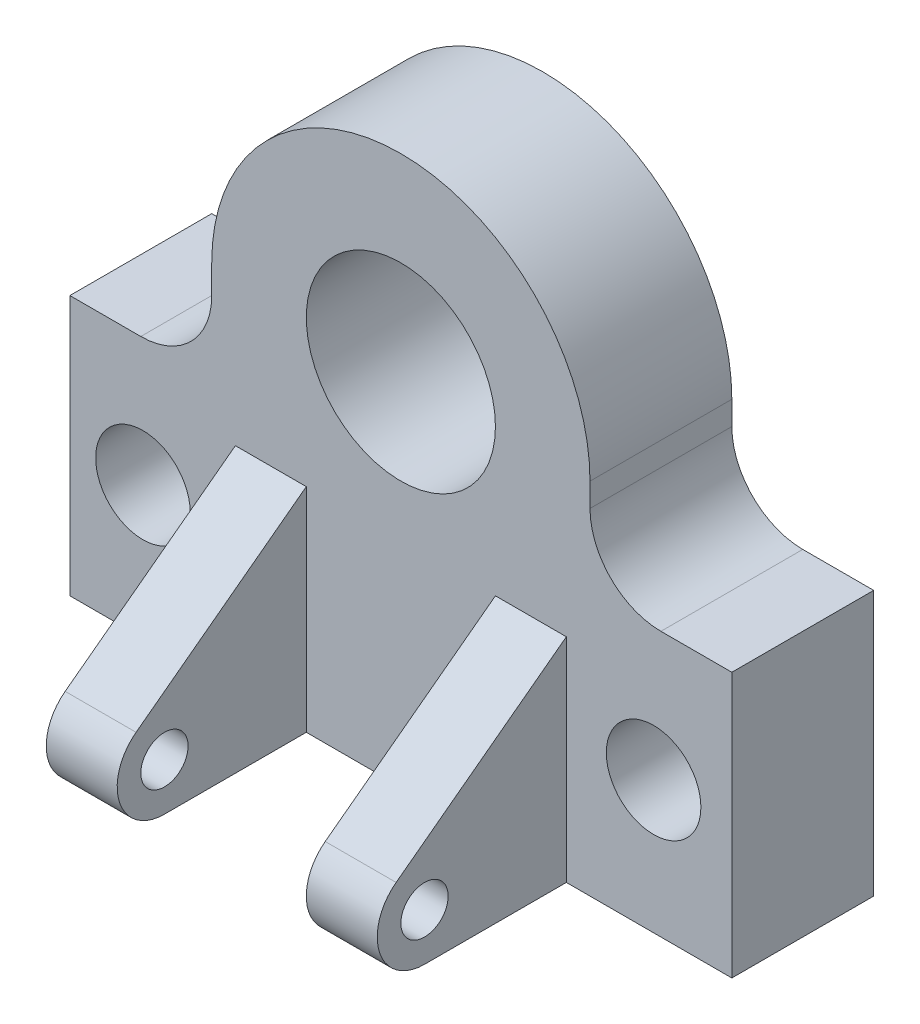
ISO-10303-21;
HEADER;
FILE_DESCRIPTION(('STEP AP214'),'2;1');
FILE_NAME('part.step','',(''),(''),'','','');
FILE_SCHEMA(('AUTOMOTIVE_DESIGN { 1 0 10303 214 1 1 1 1 }'));
ENDSEC;
DATA;
#1=APPLICATION_CONTEXT('core data for automotive mechanical design processes');
#2=APPLICATION_PROTOCOL_DEFINITION('international standard','automotive_design',2000,#1);
#3=PRODUCT_CONTEXT('',#1,'mechanical');
#4=PRODUCT('Part','Part','',(#3));
#5=PRODUCT_RELATED_PRODUCT_CATEGORY('part','',(#4));
#6=PRODUCT_DEFINITION_FORMATION('','',#4);
#7=PRODUCT_DEFINITION_CONTEXT('part definition',#1,'design');
#8=PRODUCT_DEFINITION('design','',#6,#7);
#9=PRODUCT_DEFINITION_SHAPE('','',#8);
#10=(LENGTH_UNIT() NAMED_UNIT(*) SI_UNIT(.MILLI.,.METRE.));
#11=(NAMED_UNIT(*) PLANE_ANGLE_UNIT() SI_UNIT($,.RADIAN.));
#12=(NAMED_UNIT(*) SI_UNIT($,.STERADIAN.) SOLID_ANGLE_UNIT());
#13=UNCERTAINTY_MEASURE_WITH_UNIT(LENGTH_MEASURE(1.E-05),#10,'distance_accuracy_value','');
#14=(GEOMETRIC_REPRESENTATION_CONTEXT(3) GLOBAL_UNCERTAINTY_ASSIGNED_CONTEXT((#13)) GLOBAL_UNIT_ASSIGNED_CONTEXT((#10,
#11,#12)) REPRESENTATION_CONTEXT('',''));
#15=CARTESIAN_POINT('',(0.,0.,0.));
#16=DIRECTION('',(0.,0.,1.));
#17=DIRECTION('',(1.,0.,0.));
#18=AXIS2_PLACEMENT_3D('',#15,#16,#17);
#19=CARTESIAN_POINT('',(90.,10.,60.));
#20=DIRECTION('',(1.,0.,0.));
#21=DIRECTION('',(0.,0.,-1.));
#22=AXIS2_PLACEMENT_3D('',#19,#20,#21);
#23=CYLINDRICAL_SURFACE('',#22,10.);
#24=DIRECTION('',(1.,0.,0.));
#25=VECTOR('',#24,1.);
#26=CARTESIAN_POINT('',(90.,0.,60.));
#27=LINE('',#26,#25);
#28=CARTESIAN_POINT('',(90.,0.,60.));
#29=VERTEX_POINT('',#28);
#30=CARTESIAN_POINT('',(105.,0.,60.));
#31=VERTEX_POINT('',#30);
#32=EDGE_CURVE('E179',#29,#31,#27,.T.);
#33=ORIENTED_EDGE('',*,*,#32,.T.);
#34=CARTESIAN_POINT('',(105.,10.,60.));
#35=DIRECTION('',(1.,0.,0.));
#36=DIRECTION('',(0.,0.,-1.));
#37=AXIS2_PLACEMENT_3D('',#34,#35,#36);
#38=CIRCLE('',#37,10.);
#39=CARTESIAN_POINT('',(105.,18.,66.));
#40=VERTEX_POINT('',#39);
#41=EDGE_CURVE('E167',#40,#31,#38,.T.);
#42=ORIENTED_EDGE('',*,*,#41,.F.);
#43=DIRECTION('',(1.,0.,0.));
#44=VECTOR('',#43,1.);
#45=CARTESIAN_POINT('',(90.,18.,66.));
#46=LINE('',#45,#44);
#47=CARTESIAN_POINT('',(90.,18.,66.));
#48=VERTEX_POINT('',#47);
#49=EDGE_CURVE('E178',#48,#40,#46,.T.);
#50=ORIENTED_EDGE('',*,*,#49,.F.);
#51=CARTESIAN_POINT('',(90.,10.,60.));
#52=DIRECTION('',(1.,0.,0.));
#53=DIRECTION('',(0.,0.,-1.));
#54=AXIS2_PLACEMENT_3D('',#51,#52,#53);
#55=CIRCLE('',#54,10.);
#56=EDGE_CURVE('E194',#48,#29,#55,.T.);
#57=ORIENTED_EDGE('',*,*,#56,.T.);
#58=EDGE_LOOP('',(#33,#42,#50,#57));
#59=FACE_BOUND('',#58,.T.);
#60=ADVANCED_FACE('F44',(#59),#23,.T.);
#61=CARTESIAN_POINT('',(90.,45.,30.));
#62=DIRECTION('',(0.,0.8,0.6));
#63=DIRECTION('',(0.,-0.6,0.8));
#64=AXIS2_PLACEMENT_3D('',#61,#62,#63);
#65=PLANE('',#64);
#66=ORIENTED_EDGE('',*,*,#49,.T.);
#67=DIRECTION('',(0.,-0.6,0.8));
#68=VECTOR('',#67,1.);
#69=CARTESIAN_POINT('',(105.,45.,30.));
#70=LINE('',#69,#68);
#71=CARTESIAN_POINT('',(105.,45.,30.));
#72=VERTEX_POINT('',#71);
#73=EDGE_CURVE('E170',#72,#40,#70,.T.);
#74=ORIENTED_EDGE('',*,*,#73,.F.);
#75=DIRECTION('',(1.,0.,0.));
#76=VECTOR('',#75,1.);
#77=CARTESIAN_POINT('',(90.,45.,30.));
#78=LINE('',#77,#76);
#79=CARTESIAN_POINT('',(90.,45.,30.));
#80=VERTEX_POINT('',#79);
#81=EDGE_CURVE('E190',#80,#72,#78,.T.);
#82=ORIENTED_EDGE('',*,*,#81,.F.);
#83=DIRECTION('',(0.,-0.6,0.8));
#84=VECTOR('',#83,1.);
#85=CARTESIAN_POINT('',(90.,45.,30.));
#86=LINE('',#85,#84);
#87=EDGE_CURVE('E184',#80,#48,#86,.T.);
#88=ORIENTED_EDGE('',*,*,#87,.T.);
#89=EDGE_LOOP('',(#66,#74,#82,#88));
#90=FACE_BOUND('',#89,.T.);
#91=ADVANCED_FACE('F182',(#90),#65,.T.);
#92=CARTESIAN_POINT('',(50.,10.,60.));
#93=DIRECTION('',(-1.,0.,0.));
#94=DIRECTION('',(0.,0.,1.));
#95=AXIS2_PLACEMENT_3D('',#92,#93,#94);
#96=CYLINDRICAL_SURFACE('',#95,10.);
#97=DIRECTION('',(-1.,0.,0.));
#98=VECTOR('',#97,1.);
#99=CARTESIAN_POINT('',(50.,18.,66.));
#100=LINE('',#99,#98);
#101=CARTESIAN_POINT('',(50.,18.,66.));
#102=VERTEX_POINT('',#101);
#103=CARTESIAN_POINT('',(35.,18.,66.));
#104=VERTEX_POINT('',#103);
#105=EDGE_CURVE('E232',#102,#104,#100,.T.);
#106=ORIENTED_EDGE('',*,*,#105,.T.);
#107=CARTESIAN_POINT('',(35.,10.,60.));
#108=DIRECTION('',(-1.,0.,0.));
#109=DIRECTION('',(0.,0.,1.));
#110=AXIS2_PLACEMENT_3D('',#107,#108,#109);
#111=CIRCLE('',#110,10.);
#112=CARTESIAN_POINT('',(35.,0.,60.0000000000001));
#113=VERTEX_POINT('',#112);
#114=EDGE_CURVE('E215',#113,#104,#111,.T.);
#115=ORIENTED_EDGE('',*,*,#114,.F.);
#116=DIRECTION('',(-1.,0.,0.));
#117=VECTOR('',#116,1.);
#118=CARTESIAN_POINT('',(50.,0.,60.));
#119=LINE('',#118,#117);
#120=CARTESIAN_POINT('',(50.,0.,60.));
#121=VERTEX_POINT('',#120);
#122=EDGE_CURVE('E229',#121,#113,#119,.T.);
#123=ORIENTED_EDGE('',*,*,#122,.F.);
#124=CARTESIAN_POINT('',(50.,10.,60.));
#125=DIRECTION('',(-1.,0.,0.));
#126=DIRECTION('',(0.,0.,1.));
#127=AXIS2_PLACEMENT_3D('',#124,#125,#126);
#128=CIRCLE('',#127,10.);
#129=EDGE_CURVE('E225',#121,#102,#128,.T.);
#130=ORIENTED_EDGE('',*,*,#129,.T.);
#131=EDGE_LOOP('',(#106,#115,#123,#130));
#132=FACE_BOUND('',#131,.T.);
#133=ADVANCED_FACE('F364',(#132),#96,.T.);
#134=CARTESIAN_POINT('',(50.,45.,30.));
#135=DIRECTION('',(0.,0.8,0.6));
#136=DIRECTION('',(0.,-0.6,0.8));
#137=AXIS2_PLACEMENT_3D('',#134,#135,#136);
#138=PLANE('',#137);
#139=DIRECTION('',(-1.,0.,0.));
#140=VECTOR('',#139,1.);
#141=CARTESIAN_POINT('',(50.,45.,30.));
#142=LINE('',#141,#140);
#143=CARTESIAN_POINT('',(50.,45.,30.));
#144=VERTEX_POINT('',#143);
#145=CARTESIAN_POINT('',(35.,45.,30.));
#146=VERTEX_POINT('',#145);
#147=EDGE_CURVE('E233',#144,#146,#142,.T.);
#148=ORIENTED_EDGE('',*,*,#147,.T.);
#149=DIRECTION('',(0.,0.6,-0.8));
#150=VECTOR('',#149,1.);
#151=CARTESIAN_POINT('',(35.,45.,30.));
#152=LINE('',#151,#150);
#153=EDGE_CURVE('E203',#104,#146,#152,.T.);
#154=ORIENTED_EDGE('',*,*,#153,.F.);
#155=ORIENTED_EDGE('',*,*,#105,.F.);
#156=DIRECTION('',(0.,0.6,-0.8));
#157=VECTOR('',#156,1.);
#158=CARTESIAN_POINT('',(50.,45.,30.));
#159=LINE('',#158,#157);
#160=EDGE_CURVE('E224',#102,#144,#159,.T.);
#161=ORIENTED_EDGE('',*,*,#160,.T.);
#162=EDGE_LOOP('',(#148,#154,#155,#161));
#163=FACE_BOUND('',#162,.T.);
#164=ADVANCED_FACE('F422',(#163),#138,.T.);
#165=CARTESIAN_POINT('',(0.,0.,30.));
#166=DIRECTION('',(1.,0.,0.));
#167=DIRECTION('',(0.,0.,-1.));
#168=AXIS2_PLACEMENT_3D('',#165,#166,#167);
#169=PLANE('',#168);
#170=DIRECTION('',(0.,0.,-1.));
#171=VECTOR('',#170,1.);
#172=CARTESIAN_POINT('',(0.,0.,30.));
#173=LINE('',#172,#171);
#174=CARTESIAN_POINT('',(0.,0.,30.));
#175=VERTEX_POINT('',#174);
#176=CARTESIAN_POINT('',(0.,0.,0.));
#177=VERTEX_POINT('',#176);
#178=EDGE_CURVE('E11',#175,#177,#173,.T.);
#179=ORIENTED_EDGE('',*,*,#178,.F.);
#180=DIRECTION('',(0.,-1.,0.));
#181=VECTOR('',#180,1.);
#182=CARTESIAN_POINT('',(0.,0.,30.));
#183=LINE('',#182,#181);
#184=CARTESIAN_POINT('',(0.,55.,30.));
#185=VERTEX_POINT('',#184);
#186=EDGE_CURVE('E251',#185,#175,#183,.T.);
#187=ORIENTED_EDGE('',*,*,#186,.F.);
#188=DIRECTION('',(0.,0.,-1.));
#189=VECTOR('',#188,1.);
#190=CARTESIAN_POINT('',(0.,55.,30.));
#191=LINE('',#190,#189);
#192=CARTESIAN_POINT('',(0.,55.,0.));
#193=VERTEX_POINT('',#192);
#194=EDGE_CURVE('E273',#185,#193,#191,.T.);
#195=ORIENTED_EDGE('',*,*,#194,.T.);
#196=DIRECTION('',(0.,-1.,0.));
#197=VECTOR('',#196,1.);
#198=CARTESIAN_POINT('',(0.,0.,0.));
#199=LINE('',#198,#197);
#200=EDGE_CURVE('E252',#193,#177,#199,.T.);
#201=ORIENTED_EDGE('',*,*,#200,.T.);
#202=EDGE_LOOP('',(#179,#187,#195,#201));
#203=FACE_BOUND('',#202,.T.);
#204=ADVANCED_FACE('F50',(#203),#169,.F.);
#205=CARTESIAN_POINT('',(0.,0.,30.));
#206=DIRECTION('',(0.,1.,0.));
#207=DIRECTION('',(0.,0.,1.));
#208=AXIS2_PLACEMENT_3D('',#205,#206,#207);
#209=PLANE('',#208);
#210=DIRECTION('',(0.,0.,-1.));
#211=VECTOR('',#210,1.);
#212=CARTESIAN_POINT('',(140.,0.,30.));
#213=LINE('',#212,#211);
#214=CARTESIAN_POINT('',(140.,0.,30.));
#215=VERTEX_POINT('',#214);
#216=CARTESIAN_POINT('',(140.,0.,0.));
#217=VERTEX_POINT('',#216);
#218=EDGE_CURVE('E52',#215,#217,#213,.T.);
#219=ORIENTED_EDGE('',*,*,#218,.F.);
#220=DIRECTION('',(1.,0.,0.));
#221=VECTOR('',#220,1.);
#222=CARTESIAN_POINT('',(105.,0.,30.));
#223=LINE('',#222,#221);
#224=CARTESIAN_POINT('',(105.,0.,30.));
#225=VERTEX_POINT('',#224);
#226=EDGE_CURVE('E198',#225,#215,#223,.T.);
#227=ORIENTED_EDGE('',*,*,#226,.F.);
#228=DIRECTION('',(0.,0.,-1.));
#229=VECTOR('',#228,1.);
#230=CARTESIAN_POINT('',(105.,0.,30.));
#231=LINE('',#230,#229);
#232=EDGE_CURVE('E181',#31,#225,#231,.T.);
#233=ORIENTED_EDGE('',*,*,#232,.F.);
#234=ORIENTED_EDGE('',*,*,#32,.F.);
#235=DIRECTION('',(0.,0.,-1.));
#236=VECTOR('',#235,1.);
#237=CARTESIAN_POINT('',(90.,0.,30.));
#238=LINE('',#237,#236);
#239=CARTESIAN_POINT('',(90.,0.,30.));
#240=VERTEX_POINT('',#239);
#241=EDGE_CURVE('E197',#29,#240,#238,.T.);
#242=ORIENTED_EDGE('',*,*,#241,.T.);
#243=DIRECTION('',(1.,0.,0.));
#244=VECTOR('',#243,1.);
#245=CARTESIAN_POINT('',(0.,0.,30.));
#246=LINE('',#245,#244);
#247=CARTESIAN_POINT('',(50.,0.,30.));
#248=VERTEX_POINT('',#247);
#249=EDGE_CURVE('E259',#248,#240,#246,.T.);
#250=ORIENTED_EDGE('',*,*,#249,.F.);
#251=DIRECTION('',(0.,0.,1.));
#252=VECTOR('',#251,1.);
#253=CARTESIAN_POINT('',(50.,0.,30.));
#254=LINE('',#253,#252);
#255=EDGE_CURVE('E218',#248,#121,#254,.T.);
#256=ORIENTED_EDGE('',*,*,#255,.T.);
#257=ORIENTED_EDGE('',*,*,#122,.T.);
#258=DIRECTION('',(0.,0.,1.));
#259=VECTOR('',#258,1.);
#260=CARTESIAN_POINT('',(35.,0.,30.));
#261=LINE('',#260,#259);
#262=CARTESIAN_POINT('',(35.,0.,30.));
#263=VERTEX_POINT('',#262);
#264=EDGE_CURVE('E214',#263,#113,#261,.T.);
#265=ORIENTED_EDGE('',*,*,#264,.F.);
#266=DIRECTION('',(-1.,0.,0.));
#267=VECTOR('',#266,1.);
#268=CARTESIAN_POINT('',(35.,0.,30.));
#269=LINE('',#268,#267);
#270=EDGE_CURVE('E212',#263,#175,#269,.T.);
#271=ORIENTED_EDGE('',*,*,#270,.T.);
#272=ORIENTED_EDGE('',*,*,#178,.T.);
#273=DIRECTION('',(1.,0.,0.));
#274=VECTOR('',#273,1.);
#275=CARTESIAN_POINT('',(0.,0.,0.));
#276=LINE('',#275,#274);
#277=EDGE_CURVE('E280',#177,#217,#276,.T.);
#278=ORIENTED_EDGE('',*,*,#277,.T.);
#279=EDGE_LOOP('',(#219,#227,#233,#234,#242,#250,#256,#257,#265,#271,#272,#278));
#280=FACE_BOUND('',#279,.T.);
#281=ADVANCED_FACE('F330',(#280),#209,.F.);
#282=CARTESIAN_POINT('',(140.,0.,30.));
#283=DIRECTION('',(-1.,0.,0.));
#284=DIRECTION('',(0.,0.,1.));
#285=AXIS2_PLACEMENT_3D('',#282,#283,#284);
#286=PLANE('',#285);
#287=DIRECTION('',(0.,1.,0.));
#288=VECTOR('',#287,1.);
#289=CARTESIAN_POINT('',(140.,0.,30.));
#290=LINE('',#289,#288);
#291=CARTESIAN_POINT('',(140.,56.,30.));
#292=VERTEX_POINT('',#291);
#293=EDGE_CURVE('E258',#215,#292,#290,.T.);
#294=ORIENTED_EDGE('',*,*,#293,.F.);
#295=ORIENTED_EDGE('',*,*,#218,.T.);
#296=DIRECTION('',(0.,1.,0.));
#297=VECTOR('',#296,1.);
#298=CARTESIAN_POINT('',(140.,0.,0.));
#299=LINE('',#298,#297);
#300=CARTESIAN_POINT('',(140.,56.,0.));
#301=VERTEX_POINT('',#300);
#302=EDGE_CURVE('E281',#217,#301,#299,.T.);
#303=ORIENTED_EDGE('',*,*,#302,.T.);
#304=DIRECTION('',(0.,0.,-1.));
#305=VECTOR('',#304,1.);
#306=CARTESIAN_POINT('',(140.,56.,30.));
#307=LINE('',#306,#305);
#308=EDGE_CURVE('E317',#292,#301,#307,.T.);
#309=ORIENTED_EDGE('',*,*,#308,.F.);
#310=EDGE_LOOP('',(#294,#295,#303,#309));
#311=FACE_BOUND('',#310,.T.);
#312=ADVANCED_FACE('F318',(#311),#286,.F.);
#313=CARTESIAN_POINT('',(140.,56.,30.));
#314=DIRECTION('',(0.,-1.,0.));
#315=DIRECTION('',(0.,0.,-1.));
#316=AXIS2_PLACEMENT_3D('',#313,#314,#315);
#317=PLANE('',#316);
#318=DIRECTION('',(-1.,0.,0.));
#319=VECTOR('',#318,1.);
#320=CARTESIAN_POINT('',(140.,56.,0.));
#321=LINE('',#320,#319);
#322=CARTESIAN_POINT('',(125.,56.,0.));
#323=VERTEX_POINT('',#322);
#324=EDGE_CURVE('E282',#301,#323,#321,.T.);
#325=ORIENTED_EDGE('',*,*,#324,.T.);
#326=DIRECTION('',(0.,0.,-1.));
#327=VECTOR('',#326,1.);
#328=CARTESIAN_POINT('',(125.,56.,30.));
#329=LINE('',#328,#327);
#330=CARTESIAN_POINT('',(125.,56.,30.));
#331=VERTEX_POINT('',#330);
#332=EDGE_CURVE('E312',#331,#323,#329,.T.);
#333=ORIENTED_EDGE('',*,*,#332,.F.);
#334=DIRECTION('',(-1.,0.,0.));
#335=VECTOR('',#334,1.);
#336=CARTESIAN_POINT('',(140.,56.,30.));
#337=LINE('',#336,#335);
#338=EDGE_CURVE('E261',#292,#331,#337,.T.);
#339=ORIENTED_EDGE('',*,*,#338,.F.);
#340=ORIENTED_EDGE('',*,*,#308,.T.);
#341=EDGE_LOOP('',(#325,#333,#339,#340));
#342=FACE_BOUND('',#341,.T.);
#343=ADVANCED_FACE('F340',(#342),#317,.F.);
#344=CARTESIAN_POINT('',(125.,71.,30.));
#345=DIRECTION('',(0.,0.,-1.));
#346=DIRECTION('',(-1.,0.,0.));
#347=AXIS2_PLACEMENT_3D('',#344,#345,#346);
#348=CYLINDRICAL_SURFACE('',#347,15.);
#349=CARTESIAN_POINT('',(125.,71.,0.));
#350=DIRECTION('',(0.,0.,-1.));
#351=DIRECTION('',(1.,0.,0.));
#352=AXIS2_PLACEMENT_3D('',#349,#350,#351);
#353=CIRCLE('',#352,15.);
#354=CARTESIAN_POINT('',(110.,71.,0.));
#355=VERTEX_POINT('',#354);
#356=EDGE_CURVE('E284',#323,#355,#353,.T.);
#357=ORIENTED_EDGE('',*,*,#356,.T.);
#358=DIRECTION('',(0.,0.,-1.));
#359=VECTOR('',#358,1.);
#360=CARTESIAN_POINT('',(110.,71.,30.));
#361=LINE('',#360,#359);
#362=CARTESIAN_POINT('',(110.,71.,30.));
#363=VERTEX_POINT('',#362);
#364=EDGE_CURVE('E309',#363,#355,#361,.T.);
#365=ORIENTED_EDGE('',*,*,#364,.F.);
#366=CARTESIAN_POINT('',(125.,71.,30.));
#367=DIRECTION('',(0.,0.,-1.));
#368=DIRECTION('',(1.,0.,0.));
#369=AXIS2_PLACEMENT_3D('',#366,#367,#368);
#370=CIRCLE('',#369,15.);
#371=EDGE_CURVE('E262',#331,#363,#370,.T.);
#372=ORIENTED_EDGE('',*,*,#371,.F.);
#373=ORIENTED_EDGE('',*,*,#332,.T.);
#374=EDGE_LOOP('',(#357,#365,#372,#373));
#375=FACE_BOUND('',#374,.T.);
#376=ADVANCED_FACE('F344',(#375),#348,.F.);
#377=CARTESIAN_POINT('',(110.,76.,30.));
#378=DIRECTION('',(-1.,0.,0.));
#379=DIRECTION('',(0.,0.,1.));
#380=AXIS2_PLACEMENT_3D('',#377,#378,#379);
#381=PLANE('',#380);
#382=DIRECTION('',(0.,1.,0.));
#383=VECTOR('',#382,1.);
#384=CARTESIAN_POINT('',(110.,76.,0.));
#385=LINE('',#384,#383);
#386=CARTESIAN_POINT('',(110.,76.,0.));
#387=VERTEX_POINT('',#386);
#388=EDGE_CURVE('E290',#355,#387,#385,.T.);
#389=ORIENTED_EDGE('',*,*,#388,.T.);
#390=DIRECTION('',(0.,0.,-1.));
#391=VECTOR('',#390,1.);
#392=CARTESIAN_POINT('',(110.,76.,30.));
#393=LINE('',#392,#391);
#394=CARTESIAN_POINT('',(110.,76.,30.));
#395=VERTEX_POINT('',#394);
#396=EDGE_CURVE('E310',#395,#387,#393,.T.);
#397=ORIENTED_EDGE('',*,*,#396,.F.);
#398=DIRECTION('',(0.,1.,0.));
#399=VECTOR('',#398,1.);
#400=CARTESIAN_POINT('',(110.,76.,30.));
#401=LINE('',#400,#399);
#402=EDGE_CURVE('E264',#363,#395,#401,.T.);
#403=ORIENTED_EDGE('',*,*,#402,.F.);
#404=ORIENTED_EDGE('',*,*,#364,.T.);
#405=EDGE_LOOP('',(#389,#397,#403,#404));
#406=FACE_BOUND('',#405,.T.);
#407=ADVANCED_FACE('F392',(#406),#381,.F.);
#408=CARTESIAN_POINT('',(70.,76.,30.));
#409=DIRECTION('',(0.,0.,-1.));
#410=DIRECTION('',(-1.,0.,0.));
#411=AXIS2_PLACEMENT_3D('',#408,#409,#410);
#412=CYLINDRICAL_SURFACE('',#411,40.);
#413=CARTESIAN_POINT('',(70.,76.,0.));
#414=DIRECTION('',(0.,0.,1.));
#415=DIRECTION('',(1.,0.,0.));
#416=AXIS2_PLACEMENT_3D('',#413,#414,#415);
#417=CIRCLE('',#416,40.);
#418=CARTESIAN_POINT('',(30.,76.,0.));
#419=VERTEX_POINT('',#418);
#420=EDGE_CURVE('E287',#387,#419,#417,.T.);
#421=ORIENTED_EDGE('',*,*,#420,.T.);
#422=DIRECTION('',(0.,0.,-1.));
#423=VECTOR('',#422,1.);
#424=CARTESIAN_POINT('',(30.,76.,30.));
#425=LINE('',#424,#423);
#426=CARTESIAN_POINT('',(30.,76.,30.));
#427=VERTEX_POINT('',#426);
#428=EDGE_CURVE('E302',#427,#419,#425,.T.);
#429=ORIENTED_EDGE('',*,*,#428,.F.);
#430=CARTESIAN_POINT('',(70.,76.,30.));
#431=DIRECTION('',(0.,0.,1.));
#432=DIRECTION('',(1.,0.,0.));
#433=AXIS2_PLACEMENT_3D('',#430,#431,#432);
#434=CIRCLE('',#433,40.);
#435=EDGE_CURVE('E270',#395,#427,#434,.T.);
#436=ORIENTED_EDGE('',*,*,#435,.F.);
#437=ORIENTED_EDGE('',*,*,#396,.T.);
#438=EDGE_LOOP('',(#421,#429,#436,#437));
#439=FACE_BOUND('',#438,.T.);
#440=ADVANCED_FACE('F387',(#439),#412,.T.);
#441=CARTESIAN_POINT('',(30.,70.,30.));
#442=DIRECTION('',(1.,0.,0.));
#443=DIRECTION('',(0.,1.,0.));
#444=AXIS2_PLACEMENT_3D('',#441,#442,#443);
#445=PLANE('',#444);
#446=DIRECTION('',(0.,-1.,0.));
#447=VECTOR('',#446,1.);
#448=CARTESIAN_POINT('',(30.,70.,0.));
#449=LINE('',#448,#447);
#450=CARTESIAN_POINT('',(30.,70.,0.));
#451=VERTEX_POINT('',#450);
#452=EDGE_CURVE('E293',#419,#451,#449,.T.);
#453=ORIENTED_EDGE('',*,*,#452,.T.);
#454=DIRECTION('',(0.,0.,-1.));
#455=VECTOR('',#454,1.);
#456=CARTESIAN_POINT('',(30.,70.,30.));
#457=LINE('',#456,#455);
#458=CARTESIAN_POINT('',(30.,70.,30.));
#459=VERTEX_POINT('',#458);
#460=EDGE_CURVE('E301',#459,#451,#457,.T.);
#461=ORIENTED_EDGE('',*,*,#460,.F.);
#462=DIRECTION('',(0.,-1.,0.));
#463=VECTOR('',#462,1.);
#464=CARTESIAN_POINT('',(30.,70.,30.));
#465=LINE('',#464,#463);
#466=EDGE_CURVE('E267',#427,#459,#465,.T.);
#467=ORIENTED_EDGE('',*,*,#466,.F.);
#468=ORIENTED_EDGE('',*,*,#428,.T.);
#469=EDGE_LOOP('',(#453,#461,#467,#468));
#470=FACE_BOUND('',#469,.T.);
#471=ADVANCED_FACE('F389',(#470),#445,.F.);
#472=CARTESIAN_POINT('',(15.,70.,30.));
#473=DIRECTION('',(0.,0.,-1.));
#474=DIRECTION('',(-1.,0.,0.));
#475=AXIS2_PLACEMENT_3D('',#472,#473,#474);
#476=CYLINDRICAL_SURFACE('',#475,15.);
#477=CARTESIAN_POINT('',(15.,70.,0.));
#478=DIRECTION('',(0.,0.,-1.));
#479=DIRECTION('',(1.,0.,0.));
#480=AXIS2_PLACEMENT_3D('',#477,#478,#479);
#481=CIRCLE('',#480,15.);
#482=CARTESIAN_POINT('',(15.,55.,0.));
#483=VERTEX_POINT('',#482);
#484=EDGE_CURVE('E291',#451,#483,#481,.T.);
#485=ORIENTED_EDGE('',*,*,#484,.T.);
#486=DIRECTION('',(0.,0.,-1.));
#487=VECTOR('',#486,1.);
#488=CARTESIAN_POINT('',(15.,55.,30.));
#489=LINE('',#488,#487);
#490=CARTESIAN_POINT('',(15.,55.,30.));
#491=VERTEX_POINT('',#490);
#492=EDGE_CURVE('E296',#491,#483,#489,.T.);
#493=ORIENTED_EDGE('',*,*,#492,.F.);
#494=CARTESIAN_POINT('',(15.,70.,30.));
#495=DIRECTION('',(0.,0.,-1.));
#496=DIRECTION('',(1.,0.,0.));
#497=AXIS2_PLACEMENT_3D('',#494,#495,#496);
#498=CIRCLE('',#497,15.);
#499=EDGE_CURVE('E272',#459,#491,#498,.T.);
#500=ORIENTED_EDGE('',*,*,#499,.F.);
#501=ORIENTED_EDGE('',*,*,#460,.T.);
#502=EDGE_LOOP('',(#485,#493,#500,#501));
#503=FACE_BOUND('',#502,.T.);
#504=ADVANCED_FACE('F385',(#503),#476,.F.);
#505=CARTESIAN_POINT('',(0.,55.,30.));
#506=DIRECTION('',(0.,-1.,0.));
#507=DIRECTION('',(0.,0.,-1.));
#508=AXIS2_PLACEMENT_3D('',#505,#506,#507);
#509=PLANE('',#508);
#510=DIRECTION('',(-1.,0.,0.));
#511=VECTOR('',#510,1.);
#512=CARTESIAN_POINT('',(0.,55.,0.));
#513=LINE('',#512,#511);
#514=EDGE_CURVE('E256',#483,#193,#513,.T.);
#515=ORIENTED_EDGE('',*,*,#514,.T.);
#516=ORIENTED_EDGE('',*,*,#194,.F.);
#517=DIRECTION('',(-1.,0.,0.));
#518=VECTOR('',#517,1.);
#519=CARTESIAN_POINT('',(0.,55.,30.));
#520=LINE('',#519,#518);
#521=EDGE_CURVE('E271',#491,#185,#520,.T.);
#522=ORIENTED_EDGE('',*,*,#521,.F.);
#523=ORIENTED_EDGE('',*,*,#492,.T.);
#524=EDGE_LOOP('',(#515,#516,#522,#523));
#525=FACE_BOUND('',#524,.T.);
#526=ADVANCED_FACE('F377',(#525),#509,.F.);
#527=CARTESIAN_POINT('',(15.,70.,30.));
#528=DIRECTION('',(0.,0.,1.));
#529=DIRECTION('',(1.,0.,0.));
#530=AXIS2_PLACEMENT_3D('',#527,#528,#529);
#531=PLANE('',#530);
#532=ORIENTED_EDGE('',*,*,#81,.T.);
#533=DIRECTION('',(0.,1.,0.));
#534=VECTOR('',#533,1.);
#535=CARTESIAN_POINT('',(105.,45.,30.));
#536=LINE('',#535,#534);
#537=EDGE_CURVE('E58',#225,#72,#536,.T.);
#538=ORIENTED_EDGE('',*,*,#537,.F.);
#539=ORIENTED_EDGE('',*,*,#226,.T.);
#540=ORIENTED_EDGE('',*,*,#293,.T.);
#541=ORIENTED_EDGE('',*,*,#338,.T.);
#542=ORIENTED_EDGE('',*,*,#371,.T.);
#543=ORIENTED_EDGE('',*,*,#402,.T.);
#544=ORIENTED_EDGE('',*,*,#435,.T.);
#545=ORIENTED_EDGE('',*,*,#466,.T.);
#546=ORIENTED_EDGE('',*,*,#499,.T.);
#547=ORIENTED_EDGE('',*,*,#521,.T.);
#548=ORIENTED_EDGE('',*,*,#186,.T.);
#549=ORIENTED_EDGE('',*,*,#270,.F.);
#550=DIRECTION('',(0.,-1.,0.));
#551=VECTOR('',#550,1.);
#552=CARTESIAN_POINT('',(35.,45.,30.));
#553=LINE('',#552,#551);
#554=EDGE_CURVE('E206',#146,#263,#553,.T.);
#555=ORIENTED_EDGE('',*,*,#554,.F.);
#556=ORIENTED_EDGE('',*,*,#147,.F.);
#557=DIRECTION('',(0.,-1.,0.));
#558=VECTOR('',#557,1.);
#559=CARTESIAN_POINT('',(50.,0.,30.));
#560=LINE('',#559,#558);
#561=EDGE_CURVE('E227',#144,#248,#560,.T.);
#562=ORIENTED_EDGE('',*,*,#561,.T.);
#563=ORIENTED_EDGE('',*,*,#249,.T.);
#564=DIRECTION('',(0.,1.,0.));
#565=VECTOR('',#564,1.);
#566=CARTESIAN_POINT('',(90.,0.,30.));
#567=LINE('',#566,#565);
#568=EDGE_CURVE('E67',#240,#80,#567,.T.);
#569=ORIENTED_EDGE('',*,*,#568,.T.);
#570=EDGE_LOOP('',(#532,#538,#539,#540,#541,#542,#543,#544,#545,#546,#547,#548,#549,#555,#556,
#562,#563,#569));
#571=FACE_BOUND('',#570,.T.);
#572=CARTESIAN_POINT('',(70.,76.,30.));
#573=DIRECTION('',(0.,0.,1.));
#574=DIRECTION('',(1.,0.,0.));
#575=AXIS2_PLACEMENT_3D('',#572,#573,#574);
#576=CIRCLE('',#575,20.);
#577=CARTESIAN_POINT('',(90.,76.,30.));
#578=VERTEX_POINT('',#577);
#579=EDGE_CURVE('E243',#578,#578,#576,.T.);
#580=ORIENTED_EDGE('',*,*,#579,.F.);
#581=EDGE_LOOP('',(#580));
#582=FACE_BOUND('',#581,.T.);
#583=CARTESIAN_POINT('',(15.451626978475,28.,30.));
#584=DIRECTION('',(0.,0.,1.));
#585=DIRECTION('',(1.,0.,0.));
#586=AXIS2_PLACEMENT_3D('',#583,#584,#585);
#587=CIRCLE('',#586,10.);
#588=CARTESIAN_POINT('',(25.451626978475,28.,30.));
#589=VERTEX_POINT('',#588);
#590=EDGE_CURVE('E217',#589,#589,#587,.T.);
#591=ORIENTED_EDGE('',*,*,#590,.F.);
#592=EDGE_LOOP('',(#591));
#593=FACE_BOUND('',#592,.T.);
#594=CARTESIAN_POINT('',(123.451626978475,28.,30.));
#595=DIRECTION('',(0.,0.,-1.));
#596=DIRECTION('',(-1.,0.,0.));
#597=AXIS2_PLACEMENT_3D('',#594,#595,#596);
#598=CIRCLE('',#597,9.99999999999999);
#599=CARTESIAN_POINT('',(113.451626978475,28.,30.));
#600=VERTEX_POINT('',#599);
#601=EDGE_CURVE('E192',#600,#600,#598,.F.);
#602=ORIENTED_EDGE('',*,*,#601,.F.);
#603=EDGE_LOOP('',(#602));
#604=FACE_BOUND('',#603,.T.);
#605=ADVANCED_FACE('F343',(#571,#582,#593,#604),#531,.T.);
#606=CARTESIAN_POINT('',(15.,70.,0.));
#607=DIRECTION('',(0.,0.,1.));
#608=DIRECTION('',(1.,0.,0.));
#609=AXIS2_PLACEMENT_3D('',#606,#607,#608);
#610=PLANE('',#609);
#611=CARTESIAN_POINT('',(15.451626978475,28.,0.));
#612=DIRECTION('',(0.,0.,1.));
#613=DIRECTION('',(1.,0.,0.));
#614=AXIS2_PLACEMENT_3D('',#611,#612,#613);
#615=CIRCLE('',#614,10.);
#616=CARTESIAN_POINT('',(25.451626978475,28.,0.));
#617=VERTEX_POINT('',#616);
#618=EDGE_CURVE('E239',#617,#617,#615,.T.);
#619=ORIENTED_EDGE('',*,*,#618,.T.);
#620=EDGE_LOOP('',(#619));
#621=FACE_BOUND('',#620,.T.);
#622=CARTESIAN_POINT('',(123.451626978475,28.,0.));
#623=DIRECTION('',(0.,0.,1.));
#624=DIRECTION('',(1.,0.,0.));
#625=AXIS2_PLACEMENT_3D('',#622,#623,#624);
#626=CIRCLE('',#625,9.99999999999999);
#627=CARTESIAN_POINT('',(133.451626978475,28.,0.));
#628=VERTEX_POINT('',#627);
#629=EDGE_CURVE('E234',#628,#628,#626,.T.);
#630=ORIENTED_EDGE('',*,*,#629,.T.);
#631=EDGE_LOOP('',(#630));
#632=FACE_BOUND('',#631,.T.);
#633=CARTESIAN_POINT('',(70.,76.,0.));
#634=DIRECTION('',(0.,0.,1.));
#635=DIRECTION('',(1.,0.,0.));
#636=AXIS2_PLACEMENT_3D('',#633,#634,#635);
#637=CIRCLE('',#636,20.);
#638=CARTESIAN_POINT('',(90.,76.,0.));
#639=VERTEX_POINT('',#638);
#640=EDGE_CURVE('E247',#639,#639,#637,.T.);
#641=ORIENTED_EDGE('',*,*,#640,.T.);
#642=EDGE_LOOP('',(#641));
#643=FACE_BOUND('',#642,.T.);
#644=ORIENTED_EDGE('',*,*,#200,.F.);
#645=ORIENTED_EDGE('',*,*,#514,.F.);
#646=ORIENTED_EDGE('',*,*,#484,.F.);
#647=ORIENTED_EDGE('',*,*,#452,.F.);
#648=ORIENTED_EDGE('',*,*,#420,.F.);
#649=ORIENTED_EDGE('',*,*,#388,.F.);
#650=ORIENTED_EDGE('',*,*,#356,.F.);
#651=ORIENTED_EDGE('',*,*,#324,.F.);
#652=ORIENTED_EDGE('',*,*,#302,.F.);
#653=ORIENTED_EDGE('',*,*,#277,.F.);
#654=EDGE_LOOP('',(#644,#645,#646,#647,#648,#649,#650,#651,#652,#653));
#655=FACE_BOUND('',#654,.T.);
#656=ADVANCED_FACE('F335',(#621,#632,#643,#655),#610,.F.);
#657=CARTESIAN_POINT('',(70.,76.,0.));
#658=DIRECTION('',(0.,0.,1.));
#659=DIRECTION('',(1.,0.,0.));
#660=AXIS2_PLACEMENT_3D('',#657,#658,#659);
#661=CYLINDRICAL_SURFACE('',#660,20.);
#662=ORIENTED_EDGE('',*,*,#640,.F.);
#663=EDGE_LOOP('',(#662));
#664=FACE_BOUND('',#663,.T.);
#665=ORIENTED_EDGE('',*,*,#579,.T.);
#666=EDGE_LOOP('',(#665));
#667=FACE_BOUND('',#666,.T.);
#668=ADVANCED_FACE('F432',(#664,#667),#661,.F.);
#669=CARTESIAN_POINT('',(123.451626978475,28.,0.));
#670=DIRECTION('',(0.,0.,1.));
#671=DIRECTION('',(1.,0.,0.));
#672=AXIS2_PLACEMENT_3D('',#669,#670,#671);
#673=CYLINDRICAL_SURFACE('',#672,9.99999999999999);
#674=ORIENTED_EDGE('',*,*,#629,.F.);
#675=EDGE_LOOP('',(#674));
#676=FACE_BOUND('',#675,.T.);
#677=ORIENTED_EDGE('',*,*,#601,.T.);
#678=EDGE_LOOP('',(#677));
#679=FACE_BOUND('',#678,.T.);
#680=ADVANCED_FACE('F427',(#676,#679),#673,.F.);
#681=CARTESIAN_POINT('',(15.451626978475,28.,0.));
#682=DIRECTION('',(0.,0.,1.));
#683=DIRECTION('',(1.,0.,0.));
#684=AXIS2_PLACEMENT_3D('',#681,#682,#683);
#685=CYLINDRICAL_SURFACE('',#684,10.);
#686=ORIENTED_EDGE('',*,*,#618,.F.);
#687=EDGE_LOOP('',(#686));
#688=FACE_BOUND('',#687,.T.);
#689=ORIENTED_EDGE('',*,*,#590,.T.);
#690=EDGE_LOOP('',(#689));
#691=FACE_BOUND('',#690,.T.);
#692=ADVANCED_FACE('F419',(#688,#691),#685,.F.);
#693=CARTESIAN_POINT('',(50.,10.,60.));
#694=DIRECTION('',(-1.,0.,0.));
#695=DIRECTION('',(0.,0.,1.));
#696=AXIS2_PLACEMENT_3D('',#693,#694,#695);
#697=PLANE('',#696);
#698=CARTESIAN_POINT('',(50.,10.,60.));
#699=DIRECTION('',(-1.,0.,0.));
#700=DIRECTION('',(0.,0.,1.));
#701=AXIS2_PLACEMENT_3D('',#698,#699,#700);
#702=CIRCLE('',#701,5.);
#703=CARTESIAN_POINT('',(50.,10.,65.));
#704=VERTEX_POINT('',#703);
#705=EDGE_CURVE('E199',#704,#704,#702,.T.);
#706=ORIENTED_EDGE('',*,*,#705,.T.);
#707=EDGE_LOOP('',(#706));
#708=FACE_BOUND('',#707,.T.);
#709=ORIENTED_EDGE('',*,*,#255,.F.);
#710=ORIENTED_EDGE('',*,*,#561,.F.);
#711=ORIENTED_EDGE('',*,*,#160,.F.);
#712=ORIENTED_EDGE('',*,*,#129,.F.);
#713=EDGE_LOOP('',(#709,#710,#711,#712));
#714=FACE_BOUND('',#713,.T.);
#715=ADVANCED_FACE('F363',(#708,#714),#697,.F.);
#716=CARTESIAN_POINT('',(35.,10.,60.));
#717=DIRECTION('',(-1.,0.,0.));
#718=DIRECTION('',(0.,0.,1.));
#719=AXIS2_PLACEMENT_3D('',#716,#717,#718);
#720=PLANE('',#719);
#721=CARTESIAN_POINT('',(35.,10.,60.));
#722=DIRECTION('',(-1.,0.,0.));
#723=DIRECTION('',(0.,0.,1.));
#724=AXIS2_PLACEMENT_3D('',#721,#722,#723);
#725=CIRCLE('',#724,5.);
#726=CARTESIAN_POINT('',(35.,10.,65.));
#727=VERTEX_POINT('',#726);
#728=EDGE_CURVE('E186',#727,#727,#725,.T.);
#729=ORIENTED_EDGE('',*,*,#728,.F.);
#730=EDGE_LOOP('',(#729));
#731=FACE_BOUND('',#730,.T.);
#732=ORIENTED_EDGE('',*,*,#153,.T.);
#733=ORIENTED_EDGE('',*,*,#554,.T.);
#734=ORIENTED_EDGE('',*,*,#264,.T.);
#735=ORIENTED_EDGE('',*,*,#114,.T.);
#736=EDGE_LOOP('',(#732,#733,#734,#735));
#737=FACE_BOUND('',#736,.T.);
#738=ADVANCED_FACE('F368',(#731,#737),#720,.T.);
#739=CARTESIAN_POINT('',(50.,10.,60.));
#740=DIRECTION('',(-1.,0.,0.));
#741=DIRECTION('',(0.,0.,1.));
#742=AXIS2_PLACEMENT_3D('',#739,#740,#741);
#743=CYLINDRICAL_SURFACE('',#742,5.);
#744=ORIENTED_EDGE('',*,*,#705,.F.);
#745=EDGE_LOOP('',(#744));
#746=FACE_BOUND('',#745,.T.);
#747=ORIENTED_EDGE('',*,*,#728,.T.);
#748=EDGE_LOOP('',(#747));
#749=FACE_BOUND('',#748,.T.);
#750=ADVANCED_FACE('F411',(#746,#749),#743,.F.);
#751=CARTESIAN_POINT('',(90.,10.,60.));
#752=DIRECTION('',(1.,0.,0.));
#753=DIRECTION('',(0.,0.,-1.));
#754=AXIS2_PLACEMENT_3D('',#751,#752,#753);
#755=PLANE('',#754);
#756=CARTESIAN_POINT('',(90.,10.,60.));
#757=DIRECTION('',(1.,0.,0.));
#758=DIRECTION('',(0.,0.,-1.));
#759=AXIS2_PLACEMENT_3D('',#756,#757,#758);
#760=CIRCLE('',#759,5.);
#761=CARTESIAN_POINT('',(90.,10.,55.));
#762=VERTEX_POINT('',#761);
#763=EDGE_CURVE('E708',#762,#762,#760,.T.);
#764=ORIENTED_EDGE('',*,*,#763,.T.);
#765=EDGE_LOOP('',(#764));
#766=FACE_BOUND('',#765,.T.);
#767=ORIENTED_EDGE('',*,*,#241,.F.);
#768=ORIENTED_EDGE('',*,*,#56,.F.);
#769=ORIENTED_EDGE('',*,*,#87,.F.);
#770=ORIENTED_EDGE('',*,*,#568,.F.);
#771=EDGE_LOOP('',(#767,#768,#769,#770));
#772=FACE_BOUND('',#771,.T.);
#773=ADVANCED_FACE('F354',(#766,#772),#755,.F.);
#774=CARTESIAN_POINT('',(105.,10.,60.));
#775=DIRECTION('',(1.,0.,0.));
#776=DIRECTION('',(0.,0.,-1.));
#777=AXIS2_PLACEMENT_3D('',#774,#775,#776);
#778=PLANE('',#777);
#779=CARTESIAN_POINT('',(105.,10.,60.));
#780=DIRECTION('',(1.,0.,0.));
#781=DIRECTION('',(0.,0.,-1.));
#782=AXIS2_PLACEMENT_3D('',#779,#780,#781);
#783=CIRCLE('',#782,5.);
#784=CARTESIAN_POINT('',(105.,10.,55.));
#785=VERTEX_POINT('',#784);
#786=EDGE_CURVE('E715',#785,#785,#783,.T.);
#787=ORIENTED_EDGE('',*,*,#786,.F.);
#788=EDGE_LOOP('',(#787));
#789=FACE_BOUND('',#788,.T.);
#790=ORIENTED_EDGE('',*,*,#537,.T.);
#791=ORIENTED_EDGE('',*,*,#73,.T.);
#792=ORIENTED_EDGE('',*,*,#41,.T.);
#793=ORIENTED_EDGE('',*,*,#232,.T.);
#794=EDGE_LOOP('',(#790,#791,#792,#793));
#795=FACE_BOUND('',#794,.T.);
#796=ADVANCED_FACE('F169',(#789,#795),#778,.T.);
#797=CARTESIAN_POINT('',(90.,10.,60.));
#798=DIRECTION('',(1.,0.,0.));
#799=DIRECTION('',(0.,0.,-1.));
#800=AXIS2_PLACEMENT_3D('',#797,#798,#799);
#801=CYLINDRICAL_SURFACE('',#800,5.);
#802=ORIENTED_EDGE('',*,*,#763,.F.);
#803=EDGE_LOOP('',(#802));
#804=FACE_BOUND('',#803,.T.);
#805=ORIENTED_EDGE('',*,*,#786,.T.);
#806=EDGE_LOOP('',(#805));
#807=FACE_BOUND('',#806,.T.);
#808=ADVANCED_FACE('F503',(#804,#807),#801,.F.);
#809=CLOSED_SHELL('',(#60,#91,#133,#164,#204,#281,#312,#343,#376,#407,#440,#471,#504,#526,#605,
#656,#668,#680,#692,#715,#738,#750,#773,#796,#808));
#810=MANIFOLD_SOLID_BREP('B2',#809);
#811=ADVANCED_BREP_SHAPE_REPRESENTATION('',(#18,#810),#14);
#812=SHAPE_DEFINITION_REPRESENTATION(#9,#811);
ENDSEC;
END-ISO-10303-21;
